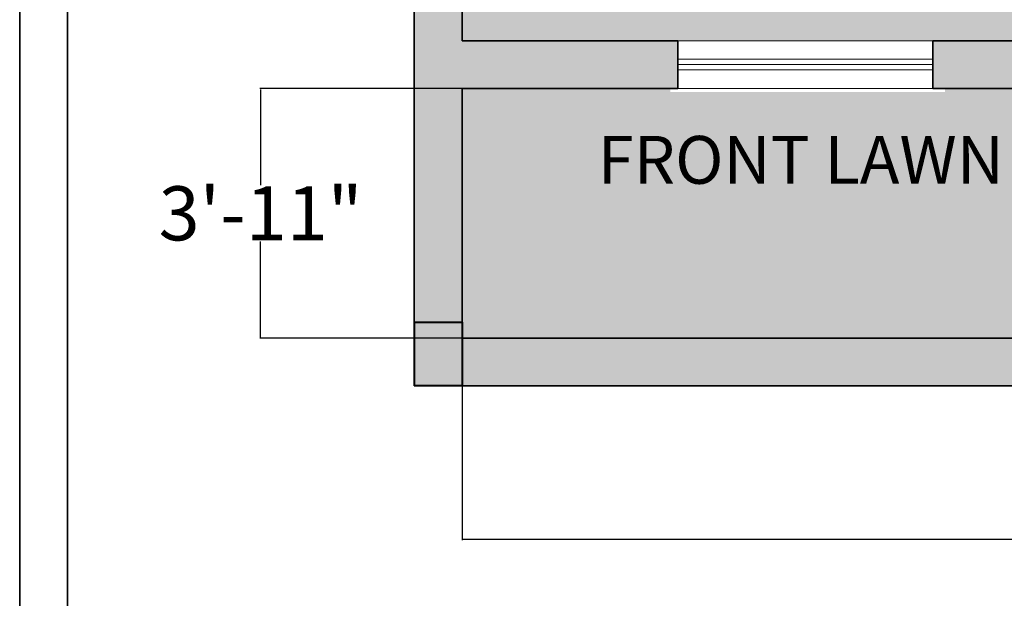
# Model space of a CAD drawing. Units: inches. Extents: x 1077 to 2505, y 1892 to 2728.
# Tile 2 of 26: x 1104 to 1290, y 2048 to 2157. Entities that reach past the tile are written whole.
import ezdxf

# ---------------------------------------------------------------- set-up
doc = ezdxf.new("R2010")
doc.units = ezdxf.units.IN
doc.linetypes.add('ACAD_ISO02W100', pattern=[15, 12, -3])
doc.layers.get('Defpoints').update_dxf_attribs({"color": 220, "linetype": 'ACAD_ISO02W100'})
for name, color, linetype, lineweight in [('A-ANNO-DIMS', 2, 'Continuous', 18), ('A-ANNO-TTLB', 7, 'Continuous', 35), ('A-AREA-IDEN', 7, 'Continuous', 18), ('A-COLS', 7, 'Continuous', 40), ('A-WALL-PATT', 7, 'Continuous', 9), ('WALL', 7, 'Continuous', 35), ('WINDOW', 160, 'Continuous', 13)]:
    doc.layers.add(name, color=color, linetype=linetype, lineweight=lineweight)
doc.layers.add('A-FLOR-PATT', color=254, linetype='Continuous', lineweight=9, true_color=0xd7ebd2)
doc.layers.add('L-PLNT-PATT', color=116, linetype='Continuous', lineweight=9, true_color=0x136734)
doc.styles.get("Standard").update_dxf_attribs({"font": 'arial.ttf'})
doc.dimstyles.get("Standard").update_dxf_attribs({"dimtxt": 10.18, "dimasz": 0.18, "dimexe": 0.18, "dimexo": 0.0625, "dimgap": 0.09, "dimtad": 0, "dimtih": 1, "dimtoh": 1, "dimdec": 0, "dimzin": 0, "dimdsep": 46, "dimlunit": 3, "dimtxsty": 'Standard', "dimcen": 0.09, "dimadec": 0, "dimazin": 0, "dimtfac": 1, "dimtdec": 0, "dimtofl": 0, "dimtmove": 0, "dimatfit": 3, "dimfxl": 1, "dimtolj": 1, "dimtzin": 0, "dimarcsym": 0})

# ---------------------------------------------------------------- blocks, each defined once
blk = doc.blocks.new('C1')
h = blk.add_hatch(color=256)
h.dxf.hatch_style = 1
h.paths.add_polyline_path([(1668.56, 2445.41), (1677.56, 2445.41), (1677.56, 2457.41), (1668.56, 2457.41)])
for p, q in [((1668.56, 2457.41), (1677.56, 2457.41)), ((1668.56, 2445.41), (1668.56, 2457.41)), ((1677.56, 2457.41), (1677.56, 2445.41)), ((1677.56, 2445.41), (1668.56, 2445.41))]:
    blk.add_line(p, q)
blk = doc.blocks.new('WINDOW-48-EXT')
for p, q in [((0, 48), (0, 0)), ((3.5, 48), (3.5, 0)), ((4.5, 48), (4.5, 0)), ((5.5, 48), (5.5, 0)), ((9, 0), (9, 48))]:
    blk.add_line(p, q)
blk = doc.blocks.new('SHEET-FRAME-RESIDENTIAL')
for points in [[(0, 830.04), (543.52, 830.04), (543.52, 0), (0, 0)], [(9, 821.04), (534.52, 821.04), (534.52, 9), (9, 9)]]:
    blk.add_lwpolyline(points, close=True)
blk = doc.blocks.new('*D65')
at = {"layer": 'A-ANNO-DIMS', "color": 0, "lineweight": -2, "transparency": 16777216}
for p, q in [((1187.53, 2097.1), (1187.53, 2059.13)), ((1432.53, 2097.1), (1432.53, 2059.13)), ((1187.71, 2059.31), (1292.37, 2059.31)), ((1432.35, 2059.31), (1327.69, 2059.31))]:
    blk.add_line(p, q, dxfattribs=at)
at = {"layer": 'A-ANNO-DIMS', "color": 0, "transparency": 16777216}
for points in [[(1187.71, 2059.34), (1187.71, 2059.28), (1187.53, 2059.31)], [(1432.35, 2059.34), (1432.35, 2059.28), (1432.53, 2059.31)]]:
    blk.add_solid(points, dxfattribs=at)
at = {"layer": 'Defpoints', "color": 0, "transparency": 16777216}
for p in [(1187.53, 2097.16), (1432.53, 2097.16), (1432.53, 2059.31)]:
    blk.add_point(p, dxfattribs=at)
at = {"layer": 'A-ANNO-DIMS', "color": 0, "transparency": 16777216, "insert": (1310.03, 2059.31), "char_height": 10.18, "attachment_point": 5}
blk.add_mtext('\\A1;20\'-5"', dxfattribs=at)
blk = doc.blocks.new('*D66')
at = {"layer": 'A-ANNO-DIMS', "color": 0, "lineweight": -2, "transparency": 16777216}
for p, q in [((1187.47, 2144.16), (1149.43, 2144.16)), ((1149.61, 2143.98), (1149.61, 2125.95)), ((1149.61, 2097.34), (1149.61, 2115.37)), ((1187.47, 2097.16), (1149.43, 2097.16))]:
    blk.add_line(p, q, dxfattribs=at)
at = {"layer": 'A-ANNO-DIMS', "color": 0, "transparency": 16777216}
for points in [[(1149.58, 2143.98), (1149.64, 2143.98), (1149.61, 2144.16)], [(1149.58, 2097.34), (1149.64, 2097.34), (1149.61, 2097.16)]]:
    blk.add_solid(points, dxfattribs=at)
at = {"layer": 'Defpoints', "color": 0, "transparency": 16777216}
for p in [(1149.61, 2144.16), (1187.53, 2144.16), (1187.53, 2097.16)]:
    blk.add_point(p, dxfattribs=at)
at = {"layer": 'A-ANNO-DIMS', "color": 0, "transparency": 16777216, "insert": (1149.61, 2120.66), "char_height": 10.18, "attachment_point": 5}
blk.add_mtext('\\A1;3\'-11"', dxfattribs=at)

msp = doc.modelspace()

# ---------------------------------------------------------------- hatches: boundary and pattern name
at = {"layer": 'A-FLOR-PATT', "transparency": 33554559}
h = msp.add_hatch(color=256, dxfattribs=at)
h.dxf.hatch_style = 1
h.paths.add_polyline_path([(1395.53, 2577.16), (1374.83, 2577.16), (1350.83, 2577.19), (1350.83, 2577.16), (1329.53, 2577.16), (1329.53, 2480.16), (1329.53, 2469.16), (1325.53, 2469.16), (1325.53, 2515.13), (1307.53, 2515.13), (1307.53, 2577.16), (1269.31, 2577.16), (1221.31, 2577.15), (1221.31, 2577.16), (1187.53, 2577.16), (1187.53, 2433.16), (1289.53, 2433.16), (1289.53, 2429.16), (1263.53, 2429.16), (1187.53, 2429.16), (1187.53, 2395.02), (1187.53, 2395.02), (1187.53, 2371.02), (1187.53, 2371.02), (1187.53, 2307.16), (1259.53, 2307.16), (1259.53, 2399.16), (1263.53, 2399.16), (1263.53, 2307.16), (1289.53, 2307.16), (1289.53, 2306.23), (1325.53, 2306.23), (1325.53, 2307.16), (1329.53, 2307.16), (1329.53, 2306.23), (1365.53, 2306.23), (1365.53, 2307.16), (1432.53, 2307.16), (1432.53, 2088.16), (1547.53, 2088.16), (1547.53, 2140.08), (1511.53, 2140.08), (1511.53, 2267.16), (1475.53, 2267.16), (1475.53, 2303.16), (1468.53, 2303.16), (1468.53, 2307.16), (1547.53, 2307.16), (1547.53, 2348.22), (1547.53, 2396.22), (1547.53, 2429.16), (1435.53, 2429.16), (1435.53, 2433.16), (1476.35, 2433.16), (1476.35, 2451.18), (1547.53, 2451.18), (1547.53, 2577.16), (1499.53, 2577.16), (1499.53, 2586.16), (1547.53, 2586.16), (1547.53, 2642.16), (1518.18, 2642.16), (1518.18, 2642.05), (1494.15, 2642.05), (1494.15, 2642.16), (1469.53, 2642.16), (1469.53, 2577.16), (1399.53, 2577.16), (1399.53, 2429.16), (1325.53, 2429.16), (1325.53, 2433.16), (1329.53, 2433.16), (1395.53, 2433.16), (1395.53, 2480.16), (1359.53, 2480.16), (1359.53, 2484.16), (1395.53, 2484.16)])
h.paths.add_polyline_path([(1357.65, 2482.07), (1355.65, 2482.07), (1355.65, 2481.07, 0.414214), (1356.65, 2480.07), (1344.65, 2480.07), (1344.65, 2477.06), (1343.27, 2477.06), (1343.27, 2480.07), (1330.65, 2480.07, -0.414214), (1329.65, 2481.07), (1329.65, 2484.07), (1331.65, 2484.07), (1331.65, 2510.07, -0.446908)], flags=16)
h.paths.add_polyline_path([(1305.09, 2559.18), (1288.89, 2559.18), (1288.89, 2575.38), (1305.09, 2575.38)], flags=16)
h.paths.add_polyline_path([(1304.19, 2560.08), (1289.79, 2560.08), (1289.79, 2574.48), (1304.19, 2574.48)], flags=0)
h.paths.add_polyline_path([(1287.99, 2500.68, -0.414214), (1287.09, 2499.78), (1265.14, 2499.78), (1224.09, 2499.78, -0.414214), (1223.19, 2500.68), (1223.19, 2557.16), (1223.19, 2571.74), (1223.19, 2575.38), (1287.99, 2575.38), (1287.99, 2571.74), (1287.09, 2571.74, -0.414214), (1287.99, 2570.84)], flags=16)
h.paths.add_polyline_path([(1292.98, 2569.05, -1), (1300.92, 2569.05, -1)], flags=0)
h.paths.add_polyline_path([(1293.32, 2569.05, -1), (1300.58, 2569.05, -1)], flags=0)
h.paths.add_polyline_path([(1322.8, 2462.21), (1322.8, 2431.71), (1323.05, 2430.71), (1323.05, 2431.71), (1321.8, 2431.71), (1321.8, 2462.19, 0.404641), (1292.3, 2431.71), (1292.05, 2430.71, -0.414214), (1291.55, 2430.21), (1291.05, 2430.21), (1291.05, 2429.71, -0.414214), (1290.55, 2429.21), (1289.55, 2429.21), (1289.55, 2434.21), (1290.55, 2434.21, -0.414214), (1291.05, 2433.71), (1291.05, 2433.21), (1291.55, 2433.21, -0.414214), (1292.05, 2432.71), (1292.3, 2431.71, -0.414214)], flags=16)
h.paths.add_polyline_path([(1287.82, 2548.28, 0.292232), (1279.17, 2536.8, 0.052719), (1223.93, 2548.28), (1223.28, 2548.28), (1223.28, 2557.16), (1223.93, 2557.16), (1245.42, 2557.16, -0.117785), (1245.77, 2557.93, -0.059418), (1254.87, 2567.02, -0.379859), (1257.28, 2566.88, -0.02509), (1261.41, 2563.32, -0.025935), (1265.65, 2567.02, -0.379859), (1268.06, 2566.88, -0.061767), (1277.52, 2557.43, -0.069393), (1277.82, 2557.16), (1287.82, 2557.16)], flags=0)
h.paths.add_polyline_path([(1263.47, 2548.28), (1260.56, 2548.28, -0.015371), (1258.01, 2546.13, -0.429576), (1255.37, 2546.06, -0.016036), (1252.69, 2548.28), (1223.28, 2548.28), (1223.28, 2554.42), (1246.78, 2554.42, 0.055344), (1255.37, 2546.06, 0.331768), (1257.52, 2545.74, 0.027343), (1262, 2549.64, 0.00919)], flags=0)
h.paths.add_polyline_path([(1295.56, 2568.34), (1296.87, 2569.09), (1296.87, 2570.6, 0.399698), (1295.39, 2569.05, 0.119004)], flags=0)
h.paths.add_polyline_path([(1295.21, 2569.05, -1), (1298.68, 2569.05, -1)], flags=0)
h.paths.add_polyline_path([(1296.95, 2568.96), (1297.03, 2569), (1297.03, 2569.09), (1296.99, 2569.11), (1296.91, 2568.98)], flags=0)
h.paths.add_polyline_path([(1402.28, 2462.19, -0.414214), (1432.78, 2431.69), (1433.03, 2432.69), (1432.78, 2431.69, 0.404641), (1403.28, 2462.17), (1403.28, 2431.69), (1402.03, 2431.69), (1402.03, 2430.69, -0.414214), (1401.53, 2430.19), (1401.03, 2430.19), (1401.03, 2429.69, -0.414214), (1400.53, 2429.19), (1399.53, 2429.19), (1399.53, 2434.19), (1400.53, 2434.19, -0.414214), (1401.03, 2433.69), (1401.03, 2433.19), (1401.53, 2433.19, -0.414214), (1402.03, 2432.69)], flags=16)
h.paths.add_polyline_path([(1470.16, 2535.21, -0.414214), (1471.06, 2536.11), (1527.54, 2536.11), (1542.12, 2536.11), (1545.76, 2536.11), (1545.76, 2471.31), (1542.12, 2471.31), (1542.12, 2472.21, -0.414214), (1541.22, 2471.31), (1471.06, 2471.31, -0.414214), (1470.16, 2472.21), (1470.16, 2494.16)], flags=16)
h.paths.add_polyline_path([(1483.07, 2536.11, 0.253465), (1480.11, 2526.15, 0.2538), (1470.15, 2523.19)], flags=16)
h.paths.add_polyline_path([(1223.19, 2512.69, 0.253465), (1233.14, 2509.74, 0.2538), (1236.1, 2499.77)], flags=16)
h.paths.add_polyline_path([(1469.77, 2578.72), (1469.77, 2581.72), (1471.77, 2581.72), (1471.77, 2607.72, -0.01951), (1473.77, 2607.68), (1473.77, 2579.72), (1473.77, 2578.72, -0.414214), (1472.77, 2577.72), (1470.77, 2577.72, -0.414214)], flags=16)
h.paths.add_polyline_path([(1382.46, 2398.13), (1395.04, 2398.13), (1395.04, 2399.74), (1382.46, 2399.74)], flags=16)
h.paths.add_polyline_path([(1379.94, 2397.18), (1379.94, 2389.82), (1380.5, 2389.82), (1380.5, 2396.05, -0.41429), (1381.06, 2396.61), (1396.47, 2396.61, -0.414213), (1397.03, 2396.05), (1397.03, 2389.82), (1397.59, 2389.82), (1397.59, 2397.18)], flags=16)
h.paths.add_polyline_path([(1263.37, 2428.14), (1263.37, 2426.14, -0.414214), (1262.37, 2425.14), (1261.37, 2425.14), (1233.41, 2425.14, 0.400854), (1259.37, 2401.04), (1259.37, 2401.14), (1261.37, 2401.14, -0.446908), (1233.37, 2427.14), (1259.37, 2427.14), (1259.37, 2429.14), (1262.37, 2429.14, -0.414214)], flags=16)
h.paths.add_polyline_path([(1404.79, 2398.13), (1417.37, 2398.13), (1417.37, 2399.74), (1404.79, 2399.74)], flags=16)
h.paths.add_polyline_path([(1402.27, 2397.18), (1404.79, 2398.13), (1417.37, 2398.13), (1419.92, 2397.18)], flags=16)
h.paths.add_polyline_path([(1432.26, 2383.16), (1432.26, 2370.59), (1433.87, 2370.59), (1433.87, 2383.16)], flags=16)
h.paths.add_polyline_path([(1431.3, 2385.69), (1423.84, 2385.69), (1423.84, 2385.13), (1430.18, 2385.13, -0.41429), (1430.74, 2384.57), (1430.74, 2369.16, -0.414237), (1430.18, 2368.6), (1423.84, 2368.6), (1423.84, 2368.03), (1431.3, 2368.03)], flags=16)
h.paths.add_polyline_path([(1417.37, 2351.16), (1417.37, 2349.54), (1418.9, 2349.54, 0.414236), (1419.92, 2350.56), (1419.92, 2352.11)], flags=16)
h.paths.add_polyline_path([(1395.04, 2351.16), (1395.04, 2349.54), (1396.58, 2349.54, 0.414235), (1397.59, 2350.56), (1397.59, 2352.11)], flags=16)
h.paths.add_polyline_path([(1366.7, 2370.05), (1365.09, 2370.05), (1365.09, 2368.52, 0.414235), (1366.11, 2367.5), (1367.66, 2367.5)], flags=16)
h.paths.add_polyline_path([(1419.36, 2359.47), (1419.36, 2353.24, -0.41419), (1418.8, 2352.68), (1403.39, 2352.68, -0.414137), (1402.83, 2353.24), (1402.83, 2359.47), (1397.03, 2359.47), (1397.03, 2353.24, -0.414189), (1396.47, 2352.68), (1381.06, 2352.68, -0.414137), (1380.5, 2353.24), (1380.5, 2359.47)], flags=16)
h.paths.add_polyline_path([(1222.29, 2559.18), (1206.09, 2559.18), (1206.09, 2575.38), (1222.29, 2575.38)], flags=16)
h.paths.add_polyline_path([(1221.39, 2560.08), (1206.99, 2560.08), (1206.99, 2574.48), (1221.39, 2574.48)], flags=0)
h.paths.add_polyline_path([(1482, 2577.72), (1482, 2580.73), (1483.38, 2580.73), (1483.38, 2577.72), (1484.77, 2577.72), (1484.77, 2574.72), (1483.38, 2574.72), (1483.38, 2577.72)], flags=16)
h.paths.add_polyline_path([(1266.37, 2415.53), (1266.37, 2414.14), (1263.37, 2414.14), (1263.37, 2415.53), (1260.36, 2415.53), (1260.36, 2416.91), (1263.37, 2416.91), (1263.37, 2415.53)], flags=16)
h.paths.add_polyline_path([(1210.26, 2569.05, -1), (1218.19, 2569.05, -1)], flags=0)
h.paths.add_polyline_path([(1210.6, 2569.05, -1), (1217.85, 2569.05, -1)], flags=0)
h.paths.add_polyline_path([(1212.84, 2568.34), (1214.15, 2569.09), (1214.15, 2570.6, 0.399698), (1212.67, 2569.05, 0.119004)], flags=0)
h.paths.add_polyline_path([(1212.49, 2569.05, -1), (1215.96, 2569.05, -1)], flags=0)
h.paths.add_polyline_path([(1214.23, 2568.96), (1214.3, 2568.91), (1214.3, 2569)], flags=0)
h.paths.add_polyline_path([(1507.18, 2480.12, 0.052719), (1518.66, 2535.36), (1518.66, 2536.01), (1527.54, 2536.01), (1527.54, 2535.36), (1527.54, 2513.88, -0.117785), (1528.31, 2513.53, -0.059418), (1537.4, 2504.43, -0.379859), (1537.26, 2502.01, -0.02509), (1533.7, 2497.89, -0.025935), (1537.4, 2493.64, -0.379859), (1537.26, 2491.23, -0.061767), (1527.8, 2481.77, -0.069393), (1527.54, 2481.47), (1527.54, 2471.47), (1518.66, 2471.47, 0.292232)], flags=0)
h.paths.add_polyline_path([(1516.43, 2503.92, -0.016036), (1518.66, 2506.6), (1518.66, 2536.01), (1524.8, 2536.01), (1524.8, 2512.51, 0.055344), (1516.43, 2503.92, 0.331768), (1516.12, 2501.77, 0.027343), (1520.01, 2497.29, 0.00919), (1518.66, 2495.82), (1518.66, 2498.73, -0.015371), (1516.5, 2501.28, -0.429576)], flags=0)
h.paths.add_polyline_path([(1499.63, 2625.5, -0.171636), (1502.82, 2631.01), (1502.82, 2633.37), (1498.68, 2633.37, -0.414214), (1497.7, 2634.36), (1497.7, 2640.66, -0.414214), (1498.68, 2641.64), (1514.82, 2641.64, -0.414214), (1515.81, 2640.66), (1515.81, 2634.36, -0.414214), (1514.82, 2633.37), (1510.69, 2633.37), (1510.69, 2631.01, -0.171636), (1513.88, 2625.5, -0.258205), (1509.31, 2614.47), (1504.19, 2614.47, -0.258205)], flags=16)
h.paths.add_polyline_path([(1501.2, 2625.5, -0.171636), (1504.39, 2631.01), (1509.12, 2631.01, -0.171636), (1512.3, 2625.5, -0.210384), (1509.35, 2616.02), (1504.16, 2616.02, -0.210384)], flags=0)
h.paths.add_polyline_path([(1529.56, 2537.01), (1529.56, 2553.21), (1545.76, 2553.21), (1545.76, 2537.01)], flags=16)
h.paths.add_polyline_path([(1530.46, 2537.91), (1530.46, 2552.31), (1544.86, 2552.31), (1544.86, 2537.91)], flags=0)
h.paths.add_polyline_path([(1535.45, 2545.07, -1), (1543.39, 2545.07, -1)], flags=0)
h.paths.add_polyline_path([(1535.8, 2545.07, -1), (1543.05, 2545.07, -1)], flags=0)
h.paths.add_polyline_path([(1529.56, 2470.41), (1545.76, 2470.41), (1545.76, 2454.21), (1529.56, 2454.21)], flags=16)
h.paths.add_polyline_path([(1541.16, 2544.99), (1540.98, 2544.99, -0.544606), (1538.71, 2543.68), (1538.62, 2543.53, 0.547962)], flags=0)
h.paths.add_polyline_path([(1530.46, 2469.51), (1544.86, 2469.51), (1544.86, 2455.11), (1530.46, 2455.11)], flags=0)
h.paths.add_polyline_path([(1539.47, 2545.14), (1539.42, 2545.22), (1539.38, 2545.14)], flags=0)
h.paths.add_polyline_path([(1543.39, 2462.34, -1), (1535.45, 2462.34, -1)], flags=0)
h.paths.add_polyline_path([(1543.05, 2462.34, -1), (1535.8, 2462.34, -1)], flags=0)
h.paths.add_polyline_path([(1541.16, 2462.27), (1540.98, 2462.27, -0.544606), (1538.71, 2460.96), (1538.62, 2460.8, 0.547962)], flags=0)
h.paths.add_polyline_path([(1539.47, 2462.42), (1539.42, 2462.5), (1539.38, 2462.42)], flags=0)
h.paths.add_polyline_path([(1435.32, 2335.25, -0.414214), (1465.82, 2304.75), (1466.07, 2305.75), (1465.82, 2304.75, 0.404641), (1436.32, 2335.23), (1436.32, 2304.75), (1435.07, 2304.75), (1435.07, 2303.75, -0.414214), (1434.57, 2303.25), (1434.07, 2303.25), (1434.07, 2302.75, -0.414214), (1433.57, 2302.25), (1432.57, 2302.25), (1432.57, 2307.25), (1433.57, 2307.25, -0.414214), (1434.07, 2306.75), (1434.07, 2306.25), (1434.57, 2306.25, -0.414214), (1435.07, 2305.75)], flags=16)
h.paths.add_polyline_path([(1532.13, 2635.71), (1535.43, 2635.71), (1535.43, 2635.89), (1532.13, 2635.89)], flags=16)
edge = h.paths.add_edge_path(flags=16)
edge.add_arc((1535.98, 2632.67), 0.183, 270, 360)
edge.add_line((1536.17, 2632.67), (1536.17, 2639.82))
edge.add_line((1536.17, 2639.82), (1538.29, 2639.82))
edge.add_line((1538.29, 2639.82), (1538.29, 2641.82))
edge.add_line((1538.29, 2641.82), (1533.25, 2641.82))
edge.add_line((1533.25, 2641.82), (1533.25, 2639.82))
edge.add_line((1533.25, 2639.82), (1534.87, 2639.82))
edge.add_line((1534.87, 2639.82), (1534.87, 2639))
edge.add_line((1534.87, 2639), (1533.7, 2639))
edge.add_line((1533.7, 2639), (1533.7, 2639.82))
edge.add_line((1533.7, 2639.82), (1533.25, 2639.82))
edge.add_line((1533.25, 2639.82), (1533.25, 2641.82))
edge.add_line((1533.25, 2641.82), (1538.29, 2641.82))
edge.add_line((1538.29, 2641.82), (1538.29, 2641.34))
edge.add_line((1538.29, 2641.34), (1540.64, 2641.58))
edge.add_line((1540.64, 2641.58), (1540.64, 2641.82))
edge.add_line((1540.64, 2641.82), (1541.5, 2641.82))
edge.add_line((1541.5, 2641.82), (1541.5, 2641.25))
edge.add_line((1541.5, 2641.25), (1541.31, 2639.79))
edge.add_ellipse((1541.09, 2638.95), major_axis=(-1.08, 0), ratio=0.790849, start_angle=180, end_angle=255.2976, ccw=False)
edge.add_line((1542.17, 2638.95), (1542.17, 2638.38))
edge.add_ellipse((1541.09, 2638.38), major_axis=(-1.08, 0), ratio=0.790849, start_angle=0, end_angle=180, ccw=False)
edge.add_line((1540, 2638.38), (1540.01, 2638.87))
edge.add_ellipse((1541.09, 2638.95), major_axis=(-1.08, 0), ratio=0.790849, start_angle=284.7024, end_angle=364.0401, ccw=False)
edge.add_line((1540.78, 2639.75), (1540.78, 2641.25))
edge.add_line((1540.78, 2641.25), (1540.64, 2641.25))
edge.add_line((1540.64, 2641.25), (1538.29, 2641.01))
edge.add_line((1538.29, 2641.01), (1538.29, 2639.82))
edge.add_line((1538.29, 2639.82), (1536.17, 2639.82))
edge.add_line((1536.17, 2639.82), (1536.17, 2632.48))
edge.add_line((1536.17, 2632.48), (1535.98, 2632.48))
h.paths.add_polyline_path([(1496.32, 2250.34, -0.292371), (1498.9, 2247.83, -0.085148), (1501.21, 2208.85, -0.01331), (1500.27, 2098.5, -0.379287), (1497.22, 2095.28, -0.0502), (1441.54, 2095.28, -0.379287), (1438.5, 2098.5, -0.01331), (1437.56, 2208.85, -0.086132), (1439.96, 2248.26, -0.295116), (1442.59, 2250.78, -0.114238)], flags=16)
h.paths.add_polyline_path([(1495.16, 2205.84, -0.355389), (1496.7, 2202.1), (1492.94, 2189.65, -0.398275), (1489.12, 2187.47, 0.113332), (1449.64, 2187.47, -0.398275), (1445.82, 2189.65), (1442.06, 2202.1, -0.355394), (1443.6, 2205.84, -0.265725)], flags=0)
h.paths.add_polyline_path([(1440.37, 2195.72), (1445.94, 2181.67), (1445.94, 2160.63), (1440.84, 2157.26)], flags=0)
h.paths.add_polyline_path([(1498.46, 2195.72), (1497.99, 2157.26), (1492.88, 2160.63), (1492.88, 2181.67)], flags=0)
h.paths.add_polyline_path([(1445.94, 2158.37), (1445.94, 2137.12), (1441.12, 2122.56), (1440.87, 2155.03)], flags=0)
h.paths.add_polyline_path([(1492.88, 2158.37), (1497.96, 2155.03), (1497.71, 2122.56), (1492.88, 2137.12)], flags=0)
h.paths.add_polyline_path([(1489.88, 2130.4), (1494.39, 2107.67, -0.090102), (1444.44, 2107.65), (1448.95, 2130.39, 0.036636)], flags=0)
h.paths.add_polyline_path([(1447.54, 2159.34), (1497.44, 2159.34), (1497.44, 2177.89), (1447.54, 2177.89)], flags=8)
h.paths.add_polyline_path([(1196.44, 2354.84), (1246.65, 2354.84), (1246.65, 2388.43), (1196.44, 2388.43)], flags=24)
h.paths.add_polyline_path([(1296.09, 2360.25), (1353.81, 2360.25), (1353.81, 2393.84), (1296.09, 2393.84)], flags=24)
h.paths.add_polyline_path([(1400.72, 2471.85), (1470.63, 2471.85), (1470.63, 2505.44), (1400.72, 2505.44)], flags=24)
h.paths.add_polyline_path([(1324.78, 2448.48), (1394.95, 2448.48), (1394.95, 2467.02), (1324.78, 2467.02)], flags=24)
h.paths.add_polyline_path([(1335.08, 2531.43), (1389.67, 2531.43), (1389.67, 2565.02), (1335.08, 2565.02)], flags=24)
h.paths.add_polyline_path([(1225.76, 2460), (1295.67, 2460), (1295.67, 2493.58), (1225.76, 2493.58)], flags=24)
h = msp.add_hatch(color=256, dxfattribs=at)
h.dxf.hatch_style = 1
h.paths.add_polyline_path([(1547.53, 2348.22), (1547.53, 2396.22), (1547.53, 2425.11), (1547.53, 2425.11), (1547.53, 2429.16), (1435.53, 2429.16), (1434.03, 2429.21), (1434.03, 2430.19), (1433.03, 2430.19), (1432.78, 2431.69, 0.404641), (1403.28, 2462.17), (1403.28, 2431.69), (1402.03, 2431.69), (1402.03, 2430.19), (1401.03, 2430.19), (1401.03, 2429.19), (1399.53, 2429.19), (1399.53, 2429.19), (1399.53, 2429.16), (1334.67, 2429.16), (1334.67, 2423.95), (1325.67, 2423.95), (1325.67, 2429.16), (1325.53, 2429.16), (1324.05, 2429.24), (1324.05, 2430.21), (1323.05, 2430.21), (1323.05, 2431.71), (1321.8, 2431.71), (1321.8, 2462.19, 0.416544), (1292.05, 2430.73, -0.423614), (1291.55, 2430.21), (1291.05, 2430.21), (1291.05, 2429.21), (1289.55, 2429.21), (1289.53, 2429.21), (1289.53, 2429.16), (1263.37, 2429.16), (1263.37, 2415.53), (1266.37, 2415.53), (1266.37, 2414.14), (1263.37, 2414.14), (1263.37, 2399.16), (1263.53, 2399.16), (1263.53, 2307.16), (1289.53, 2307.16), (1289.53, 2306.23), (1323.26, 2306.23), (1323.26, 2307.21), (1332.26, 2307.21), (1365.53, 2306.23), (1365.53, 2307.16), (1432.53, 2307.16), (1432.57, 2307.16), (1432.57, 2307.25), (1434.07, 2307.25), (1434.07, 2306.25), (1435.32, 2306.25), (1435.32, 2335.25, -0.407346), (1466.07, 2305.73, -0.423614), (1466.57, 2306.25), (1467.07, 2306.25), (1467.07, 2307.25), (1468.57, 2307.25), (1547.53, 2307.16), (1547.53, 2307.2)])
h.paths.add_polyline_path([(1430.74, 2369.16), (1430.74, 2384.57, 0.41429), (1430.18, 2385.13), (1423.84, 2385.13), (1423.84, 2368.6), (1430.18, 2368.6, 0.414237)], flags=16)
h.paths.add_polyline_path([(1432.26, 2383.16), (1432.26, 2370.59), (1433.87, 2370.59), (1433.87, 2383.16)], flags=16)
h.paths.add_polyline_path([(1431.3, 2368.03), (1431.3, 2385.69), (1432.26, 2383.16), (1432.26, 2370.59)], flags=16)
h.paths.add_polyline_path([(1417.37, 2351.16), (1417.37, 2349.54), (1418.9, 2349.54, 0.414236), (1419.92, 2350.56), (1419.92, 2352.11)], flags=16)
h.paths.add_polyline_path([(1403.39, 2352.68), (1418.78, 2352.68, 0.42427), (1419.36, 2353.24), (1419.36, 2359.47), (1402.83, 2359.47), (1402.83, 2353.24, 0.414137)], flags=16)
h.paths.add_polyline_path([(1366.7, 2370.05), (1365.09, 2370.05), (1365.09, 2368.52, 0.414235), (1366.11, 2367.5), (1367.66, 2367.5)], flags=16)
h.paths.add_polyline_path([(1382.46, 2398.13), (1395.04, 2398.13), (1395.04, 2399.74), (1382.46, 2399.74)], flags=16)
h.paths.add_polyline_path([(1396.47, 2396.61), (1381.06, 2396.61, 0.41429), (1380.5, 2396.05), (1380.5, 2389.82), (1397.03, 2389.82), (1397.03, 2396.05, 0.414213)], flags=16)
h.paths.add_polyline_path([(1402.27, 2397.18), (1402.83, 2396.05, -0.414213), (1403.39, 2396.61)], flags=16)
h.paths.add_polyline_path([(1418.8, 2396.61), (1419.36, 2396.61), (1419.36, 2396.05, 0.414237)], flags=16)
h.paths.add_polyline_path([(1404.79, 2398.13), (1417.37, 2398.13), (1417.37, 2399.74), (1404.79, 2399.74)], flags=16)
h.paths.add_polyline_path([(1381.06, 2352.68, -0.414213), (1380.5, 2353.24), (1380.27, 2352.11)], flags=16)
h.paths.add_polyline_path([(1396.58, 2349.54), (1396.58, 2349.54), (1395.04, 2349.54), (1395.04, 2349.54), (1382.46, 2349.54), (1382.46, 2351.16), (1395.04, 2351.16), (1397.59, 2352.11), (1397.59, 2350.56, -0.414235)], flags=16)
h.paths.add_polyline_path([(1379.94, 2397.18), (1382.46, 2398.13), (1395.04, 2398.13), (1397.59, 2397.18)], flags=16)
h.paths.add_polyline_path([(1368.78, 2384.59, 0.414213), (1368.22, 2384.03), (1367.66, 2367.5), (1367.66, 2385.15)], flags=16)
h.paths.add_polyline_path([(1547.53, 2574.38), (1547.51, 2574.38), (1547.51, 2577.16), (1499.53, 2577.16), (1484.77, 2577.44), (1484.77, 2574.72), (1483.38, 2574.72), (1483.38, 2577.72), (1482, 2577.72), (1469.53, 2577.72), (1469.53, 2577.16), (1401.95, 2577.16), (1401.95, 2574.12), (1399.53, 2574.12), (1399.53, 2434.19), (1401.03, 2434.19), (1401.03, 2433.19), (1402.28, 2433.19), (1402.28, 2462.19, -0.407346), (1433.03, 2432.67, -0.423614), (1433.53, 2433.19), (1434.03, 2433.19), (1434.03, 2434.19), (1435.53, 2434.19), (1476.35, 2433.81), (1476.35, 2451.18), (1547.53, 2451.18)])
h.paths.add_polyline_path([(1470.16, 2535.21, -0.414214), (1471.06, 2536.11), (1527.54, 2536.11), (1542.12, 2536.11), (1545.76, 2536.11), (1545.76, 2471.31), (1542.12, 2471.31), (1542.12, 2472.21, -0.414214), (1541.22, 2471.31), (1471.06, 2471.31, -0.414214), (1470.16, 2472.21), (1470.16, 2494.16)], flags=16)
h.paths.add_polyline_path([(1483.07, 2536.11, 0.253465), (1480.11, 2526.15, 0.2538), (1470.15, 2523.19)], flags=16)
h.paths.add_polyline_path([(1525.55, 2481.52, -0.000893), (1524.8, 2482.24), (1524.8, 2471.47), (1527.54, 2471.47), (1527.54, 2472.12), (1527.54, 2481.47, -0.388819)], flags=0)
h.paths.add_polyline_path([(1518.66, 2536.01), (1527.54, 2536.01), (1527.54, 2535.36), (1527.54, 2513.88, -0.117785), (1528.31, 2513.53, -0.059418), (1537.4, 2504.43, -0.379859), (1537.26, 2502.01, -0.02509), (1533.7, 2497.89, 0.033431), (1528.3, 2502.74, 0.308459), (1526.25, 2502.88, 0.047827), (1518.66, 2495.82), (1518.66, 2498.73, -0.015371), (1516.5, 2501.28, -0.429576), (1516.43, 2503.92, -0.016036), (1518.66, 2506.6)], flags=0)
h.paths.add_polyline_path([(1529.56, 2537.01), (1529.56, 2553.21), (1545.76, 2553.21), (1545.76, 2537.01)], flags=16)
h.paths.add_polyline_path([(1530.46, 2537.91), (1530.46, 2552.31), (1544.86, 2552.31), (1544.86, 2537.91)], flags=0)
h.paths.add_polyline_path([(1535.8, 2545.07, -1), (1543.05, 2545.07, -1)], flags=0)
h.paths.add_polyline_path([(1541.16, 2544.99), (1540.98, 2544.99, -0.544606), (1538.71, 2543.68), (1538.62, 2543.53, 0.547962)], flags=0)
h.paths.add_polyline_path([(1539.47, 2545.14), (1539.42, 2545.22), (1539.38, 2545.14)], flags=0)
h.paths.add_polyline_path([(1529.56, 2470.41), (1545.76, 2470.41), (1545.76, 2454.21), (1529.56, 2454.21)], flags=16)
h.paths.add_polyline_path([(1530.46, 2469.51), (1544.86, 2469.51), (1544.86, 2455.11), (1530.46, 2455.11)], flags=0)
h.paths.add_polyline_path([(1535.8, 2462.34, -1), (1543.05, 2462.34, -1)], flags=0)
h.paths.add_polyline_path([(1541.16, 2462.27), (1540.98, 2462.27, -0.544606), (1538.71, 2460.96), (1538.62, 2460.8, 0.547962)], flags=0)
h.paths.add_polyline_path([(1539.47, 2462.42), (1539.42, 2462.5), (1539.38, 2462.42)], flags=0)
h.paths.add_polyline_path([(1395.53, 2574.12), (1392.95, 2574.12), (1392.95, 2577.16), (1374.83, 2577.16), (1350.83, 2577.19), (1350.83, 2577.16), (1332.07, 2577.16), (1332.07, 2574), (1329.53, 2574), (1329.53, 2484.07), (1331.65, 2484.07), (1331.65, 2510.07, -0.423677), (1357.76, 2484.07), (1359.53, 2484.07), (1359.53, 2484.16), (1395.53, 2484.16)], flags=17)
h.paths.add_polyline_path([(1395.53, 2480.16), (1359.06, 2480.16, 0.437533), (1359.53, 2481.55), (1359.53, 2484.16), (1395.53, 2484.16), (1395.53, 2574.12), (1392.95, 2574.12), (1392.95, 2577.16), (1374.83, 2577.16), (1350.83, 2577.19), (1350.83, 2577.16), (1332.07, 2577.16), (1332.07, 2574), (1329.53, 2574), (1329.53, 2484.07), (1329.65, 2484.07), (1329.65, 2481.07), (1329.53, 2480.16), (1329.53, 2469.16), (1325.53, 2469.16), (1325.53, 2515.13), (1307.53, 2515.13), (1307.53, 2577.16), (1269.31, 2577.16), (1221.31, 2577.15), (1221.31, 2577.16), (1187.61, 2577.16), (1187.61, 2574.03), (1187.53, 2433.16), (1289.55, 2433.16), (1289.55, 2434.21), (1291.05, 2434.21), (1291.05, 2433.21), (1292.05, 2433.21), (1292.3, 2431.71, -0.414214), (1322.8, 2462.21), (1323.05, 2432.71, -0.414214), (1323.55, 2433.21), (1324.05, 2433.21), (1324.05, 2434.21), (1325.67, 2434.21), (1325.67, 2435.95), (1334.67, 2435.95), (1334.67, 2433.16), (1395.53, 2433.16)])
h.paths.add_polyline_path([(1344.65, 2480.07), (1344.65, 2477.06), (1343.27, 2477.06), (1343.27, 2480.07), (1332.65, 2480.07, 0.414214), (1333.65, 2481.07), (1333.65, 2482.07), (1331.65, 2482.07), (1331.65, 2484.07), (1331.65, 2510.07, -0.446908), (1357.65, 2482.07), (1355.65, 2482.07), (1355.65, 2481.07, 0.414214), (1356.65, 2480.07)], flags=16)
h.paths.add_polyline_path([(1287.99, 2500.68, -0.414214), (1287.09, 2499.78), (1265.14, 2499.78), (1224.09, 2499.78, -0.414214), (1223.19, 2500.68), (1223.19, 2557.16), (1223.19, 2571.74), (1223.19, 2575.38), (1287.99, 2575.38), (1287.99, 2571.74), (1287.09, 2571.74, -0.414214), (1287.99, 2570.84)], flags=16)
h.paths.add_polyline_path([(1277.77, 2555.17, -0.000893), (1277.05, 2554.42), (1287.82, 2554.42), (1287.82, 2557.16), (1287.17, 2557.16), (1277.82, 2557.16, -0.388819)], flags=0)
h.paths.add_polyline_path([(1223.28, 2548.28), (1223.28, 2557.16), (1223.93, 2557.16), (1245.42, 2557.16, -0.117785), (1245.77, 2557.93, -0.059418), (1254.87, 2567.02, -0.379859), (1257.28, 2566.88, -0.02509), (1261.41, 2563.32, 0.033431), (1256.55, 2557.93, 0.308459), (1256.41, 2555.88, 0.047827), (1263.47, 2548.28), (1260.56, 2548.28, -0.015371), (1258.01, 2546.13, -0.429576), (1255.37, 2546.06, -0.016036), (1252.69, 2548.28)], flags=0)
h.paths.add_polyline_path([(1305.09, 2559.18), (1288.89, 2559.18), (1288.89, 2575.38), (1305.09, 2575.38)], flags=16)
h.paths.add_polyline_path([(1304.19, 2560.08), (1289.79, 2560.08), (1289.79, 2574.48), (1304.19, 2574.48)], flags=0)
h.paths.add_polyline_path([(1300.58, 2569.05, -1), (1293.32, 2569.05, -1)], flags=0)
h.paths.add_polyline_path([(1223.19, 2512.69, 0.253465), (1233.14, 2509.74, 0.2538), (1236.1, 2499.77)], flags=16)
h.paths.add_polyline_path([(1295.56, 2568.34), (1296.87, 2569.09), (1296.87, 2570.6, 0.399698), (1295.39, 2569.05, 0.119004)], flags=0)
h.paths.add_polyline_path([(1295.21, 2569.05, -1), (1298.68, 2569.05, -1)], flags=0)
h.paths.add_polyline_path([(1296.95, 2568.96), (1297.03, 2569), (1297.03, 2569.09), (1296.99, 2569.11), (1296.91, 2568.98)], flags=0)
h.paths.add_polyline_path([(1222.29, 2559.18), (1206.09, 2559.18), (1206.09, 2575.38), (1222.29, 2575.38)], flags=16)
h.paths.add_polyline_path([(1221.39, 2560.08), (1206.99, 2560.08), (1206.99, 2574.48), (1221.39, 2574.48)], flags=0)
h.paths.add_polyline_path([(1217.85, 2569.05, -1), (1210.6, 2569.05, -1)], flags=0)
h.paths.add_polyline_path([(1212.84, 2568.34), (1214.15, 2569.09), (1214.15, 2570.6, 0.399698), (1212.67, 2569.05, 0.119004)], flags=0)
h.paths.add_polyline_path([(1212.49, 2569.05, -1), (1215.96, 2569.05, -1)], flags=0)
h.paths.add_polyline_path([(1214.23, 2568.96), (1214.3, 2569), (1214.3, 2569.09), (1214.26, 2569.11), (1214.19, 2568.98)], flags=0)
h.paths.add_polyline_path([(1259.53, 2399.14), (1259.37, 2399.14), (1259.37, 2401.04, -0.423677), (1233.37, 2427.14), (1259.37, 2427.14), (1259.37, 2429.16), (1187.53, 2429.16), (1187.53, 2395.02), (1187.53, 2395.02), (1187.53, 2371.02), (1187.53, 2371.02), (1187.53, 2311.49), (1187.55, 2311.49), (1187.55, 2307.16), (1259.53, 2307.16)])
h.paths.add_polyline_path([(1323.26, 2295.21), (1323.26, 2304.23), (1289.53, 2304.23), (1289.53, 2303.16), (1187.55, 2303.16), (1187.55, 2299.49), (1178.53, 2299.49), (1178.53, 2267.66), (1178.53, 2219.66), (1182.03, 2219.66), (1182.03, 2267.67), (1184.03, 2267.67), (1184.03, 2219.66), (1187.53, 2219.66), (1187.53, 2153.16), (1228.13, 2153.16), (1276.13, 2153.16), (1276.13, 2153.16), (1324.54, 2153.16), (1324.54, 2154.67), (1325.54, 2154.67), (1325.54, 2155.92), (1296.54, 2155.92, -0.407346), (1326.06, 2186.67, -0.423614), (1325.54, 2187.17), (1325.54, 2187.67), (1324.54, 2187.67), (1324.54, 2189.17), (1325.43, 2295.21)])
h.paths.add_polyline_path([(1432.53, 2307.16), (1365.53, 2307.16), (1365.53, 2306.23), (1365.53, 2303.16), (1428.53, 2303.16), (1428.53, 2221.2), (1428.57, 2221.2), (1428.57, 2197.2), (1428.53, 2197.16), (1428.53, 2303.01), (1404.46, 2303.01), (1404.46, 2221.2), (1329.53, 2221.2), (1329.53, 2307.16), (1325.53, 2307.16), (1325.53, 2295.21), (1325.43, 2295.21), (1324.54, 2189.17), (1324.54, 2187.67), (1326.04, 2187.67, 1.016365), (1326.06, 2186.67, 0.407348), (1296.54, 2155.92), (1325.54, 2155.92), (1325.54, 2154.67), (1324.54, 2154.67), (1324.54, 2153.16), (1329.53, 2153.16), (1329.53, 2144.16), (1432.53, 2144.16)])
h.paths.add_polyline_path([(1361.95, 2194.26), (1361.95, 2193.16), (1329.53, 2193.16), (1329.53, 2189.16), (1329.54, 2188.17), (1329.54, 2189.16), (1329.53, 2189.16), (1329.53, 2193.16), (1361.95, 2193.16), (1361.95, 2196.26), (1409.95, 2196.26), (1409.95, 2194.26)], flags=16)
h.paths.add_polyline_path([(1377.02, 2200.5), (1345.91, 2200.5), (1345.91, 2218.4), (1347.87, 2218.4), (1347.87, 2219.18), (1374.75, 2219.18), (1374.75, 2218.4), (1377.02, 2218.4)], flags=16)
h.paths.add_polyline_path([(1367.07, 2210.7, -1), (1373.34, 2210.7, -1)], flags=0)
h.paths.add_polyline_path([(1349.92, 2210.7, -1), (1356.98, 2210.7, -1)], flags=0)
h.paths.add_polyline_path([(1405.95, 2256.57), (1405.95, 2277.6), (1427.86, 2277.6), (1427.86, 2256.57)], flags=16)
h.paths.add_polyline_path([(1412.92, 2258.68, -0.414201), (1410.93, 2260.67), (1410.93, 2273.62, -0.414239), (1412.92, 2275.61), (1423.88, 2275.61, -0.414227), (1425.87, 2273.62), (1425.87, 2260.67, -0.414214), (1423.88, 2258.68)], flags=0)
h.paths.add_polyline_path([(1407.61, 2263.66, -1), (1409.18, 2263.66, -1)], flags=0)
h.paths.add_polyline_path([(1407.61, 2267.14, -1), (1409.18, 2267.14, -1)], flags=0)
h.paths.add_polyline_path([(1416.91, 2267.15, -1), (1419.89, 2267.15, -1)], flags=0)
h.paths.add_polyline_path([(1407.61, 2270.63, -1), (1409.18, 2270.63, -1)], flags=0)
h.paths.add_polyline_path([(1475.53, 2303.16), (1468.57, 2303.16), (1468.57, 2302.25), (1467.07, 2302.25), (1467.07, 2303.25), (1466.07, 2303.25), (1465.82, 2304.75, 0.404641), (1436.32, 2335.23), (1436.32, 2304.75), (1435.07, 2304.75), (1435.07, 2303.25), (1434.07, 2303.25), (1434.07, 2302.25), (1432.53, 2302.25), (1432.53, 2144.16), (1432.53, 2088.16), (1547.52, 2088.16), (1547.52, 2100.19), (1547.52, 2140.08), (1511.53, 2140.08), (1511.53, 2267.16), (1475.53, 2267.16)])
h.paths.add_polyline_path([(1438.35, 2102.86, 0.033498), (1438.37, 2102.21, -0.000079)], flags=16)
h.paths.add_polyline_path([(1496.32, 2250.34, -0.292371), (1498.9, 2247.83, -0.085148), (1501.21, 2208.85, -0.012784), (1500.42, 2102.86, -0.033498), (1500.39, 2102.21, 0.012863), (1501.21, 2208.85, 0.077283), (1499.67, 2244.3, 0.265882), (1497.48, 2246.8, 0.14401), (1441.46, 2247.36, 0.270646), (1439.21, 2244.85, -0.007564), (1439.96, 2248.26, -0.295116), (1442.59, 2250.78, -0.114238)], flags=16)
h.paths.add_polyline_path([(1495.16, 2205.84, -0.355389), (1496.7, 2202.1), (1492.94, 2189.65, -0.398275), (1489.12, 2187.47, 0.113332), (1449.64, 2187.47, -0.398275), (1445.82, 2189.65), (1442.06, 2202.1, -0.355394), (1443.6, 2205.84, -0.265725)], flags=16)
h.paths.add_polyline_path([(1440.37, 2195.72), (1445.94, 2181.67), (1445.94, 2160.63), (1440.84, 2157.26)], flags=16)
h.paths.add_polyline_path([(1498.46, 2195.72), (1497.99, 2157.26), (1492.88, 2160.63), (1492.88, 2181.67)], flags=16)
h.paths.add_polyline_path([(1445.94, 2158.37), (1445.94, 2137.12), (1441.12, 2122.56), (1440.87, 2155.03)], flags=16)
h.paths.add_polyline_path([(1492.88, 2158.37), (1497.96, 2155.03), (1497.71, 2122.56), (1492.88, 2137.12)], flags=16)
h.paths.add_polyline_path([(1489.88, 2130.4), (1494.39, 2107.67, -0.090102), (1444.44, 2107.65), (1448.95, 2130.39, 0.036636)], flags=16)
h.paths.add_polyline_path([(1296.09, 2360.25), (1353.81, 2360.25), (1353.81, 2393.84), (1296.09, 2393.84)], flags=24)
h.paths.add_polyline_path([(1400.72, 2471.85), (1470.63, 2471.85), (1470.63, 2505.44), (1400.72, 2505.44)], flags=24)
h.paths.add_polyline_path([(1335.08, 2531.43), (1389.67, 2531.43), (1389.67, 2565.02), (1335.08, 2565.02)], flags=24)
h.paths.add_polyline_path([(1324.78, 2448.48), (1394.95, 2448.48), (1394.95, 2467.02), (1324.78, 2467.02)], flags=24)
h.paths.add_polyline_path([(1225.76, 2460), (1295.67, 2460), (1295.67, 2493.58), (1225.76, 2493.58)], flags=24)
h.paths.add_polyline_path([(1196.44, 2354.84), (1246.65, 2354.84), (1246.65, 2388.43), (1196.44, 2388.43)], flags=24)
h.paths.add_polyline_path([(1447.54, 2159.34), (1497.44, 2159.34), (1497.44, 2177.89), (1447.54, 2177.89)], flags=24)
at = {"layer": 'A-WALL-PATT', "transparency": 33554585}
h = msp.add_hatch(color=256, dxfattribs=at)
h.dxf.hatch_style = 1
h.paths.add_polyline_path([(1187.53, 2424), (1178.53, 2424), (1178.53, 2395.02), (1187.53, 2395.02)])
h.paths.add_polyline_path([(1187.53, 2371.02), (1178.53, 2371.02), (1178.53, 2311.49), (1187.53, 2311.49)])
h.paths.add_polyline_path([(1228.13, 2153.16), (1187.53, 2153.16), (1187.53, 2219.66), (1178.53, 2219.66), (1178.53, 2100.18), (1187.53, 2100.18), (1187.53, 2144.16), (1228.13, 2144.16)])
h.paths.add_polyline_path([(1432.53, 2097.16), (1187.53, 2097.16), (1187.53, 2100.18), (1178.53, 2100.18), (1178.53, 2088.16), (1432.53, 2088.16)])
h.paths.add_polyline_path([(1556.53, 2348.22), (1547.53, 2348.22), (1547.53, 2348.22), (1547.53, 2307.16), (1468.53, 2307.16), (1468.53, 2303.16), (1547.53, 2303.16), (1547.53, 2088.16), (1556.53, 2088.16)])
h.paths.add_polyline_path([(1556.53, 2425.11), (1547.53, 2425.11), (1547.53, 2396.22), (1556.53, 2396.22)])
h.paths.add_polyline_path([(1547.53, 2433.16), (1435.53, 2433.16), (1435.53, 2429.16), (1547.53, 2429.16)])
h.paths.add_polyline_path([(1556.53, 2574.38), (1547.53, 2574.38), (1547.53, 2451.18), (1547.55, 2451.18), (1547.55, 2437.11), (1556.53, 2437.11)])
h.paths.add_polyline_path([(1556.53, 2639.11), (1547.53, 2639.11), (1547.53, 2586.38), (1556.53, 2586.38)])
h.paths.add_polyline_path([(1556.53, 2639.11), (1547.53, 2639.11), (1547.53, 2642.16), (1518.18, 2642.16), (1518.18, 2642.05), (1494.18, 2642.05), (1494.18, 2651.05), (1518.15, 2651.05), (1518.15, 2651.16), (1556.53, 2651.16)])
h.paths.add_polyline_path([(1494.15, 2651.16), (1469.6, 2651.16), (1469.6, 2642.16), (1494.15, 2642.16)])
h.paths.add_polyline_path([(1221.31, 2577.16), (1187.61, 2577.16), (1187.61, 2574.03), (1178.61, 2574.03), (1178.61, 2586.16), (1221.31, 2586.16)])
h.paths.add_polyline_path([(1323.07, 2586.16), (1269.31, 2586.16), (1269.31, 2577.16), (1323.07, 2577.16)])
h.paths.add_polyline_path([(1374.84, 2586.19), (1374.84, 2577.19), (1350.84, 2577.19), (1350.83, 2577.19), (1350.83, 2577.16), (1332.07, 2577.16), (1332.07, 2574), (1323.07, 2574), (1323.07, 2586.16), (1350.83, 2586.16), (1350.84, 2586.16), (1350.84, 2586.19)])
h.paths.add_polyline_path([(1392.95, 2586.16), (1374.84, 2586.16), (1374.84, 2577.16), (1392.95, 2577.16)], flags=17)
h.paths.add_polyline_path([(1469.53, 2642.16), (1469.6, 2651.16), (1460.53, 2651.16), (1460.53, 2586.16), (1392.95, 2586.16), (1392.95, 2577.16), (1395.53, 2577.16), (1395.53, 2484.16), (1359.53, 2484.16), (1359.53, 2480.16), (1395.53, 2480.16), (1395.53, 2433.16), (1329.53, 2433.16), (1325.53, 2433.16), (1325.53, 2429.16), (1399.53, 2429.16), (1399.53, 2577.16), (1469.53, 2577.16)])
h.paths.add_polyline_path([(1187.53, 2574.03), (1178.53, 2574.03), (1178.53, 2436), (1187.53, 2436)])
at = {"layer": 'A-WALL-PATT', "transparency": 33554559}
h = msp.add_hatch(color=256, dxfattribs=at)
h.dxf.hatch_style = 1
h.paths.add_polyline_path([(1289.53, 2433.16), (1187.46, 2433.16), (1187.46, 2429.16), (1263.53, 2429.16), (1289.53, 2429.16)])
h.paths.add_polyline_path([(1329.53, 2574), (1325.53, 2574), (1325.53, 2469.16), (1329.53, 2469.16), (1329.53, 2480.16)])
h.paths.add_polyline_path([(1547.51, 2586.16), (1499.53, 2586.16), (1499.53, 2581.72), (1499.77, 2581.72), (1499.77, 2578.72, -0.178139), (1499.53, 2578.07), (1499.53, 2577.16), (1547.51, 2577.16)])
h.paths.add_polyline_path([(1329.53, 2153.16), (1276.13, 2153.16), (1276.13, 2144.16), (1329.53, 2144.16)])
at = {"layer": 'L-PLNT-PATT', "transparency": 33554610}
h = msp.add_hatch(color=256, dxfattribs=at)
h.dxf.hatch_style = 1
h.paths.add_polyline_path([(1430.86, 2144.16), (1278.41, 2144.16), (1278.41, 2143.5), (1226.73, 2143.5), (1226.73, 2144.16), (1187.53, 2144.16), (1187.53, 2100.18), (1187.54, 2100.18), (1187.54, 2097.16), (1423.5, 2097.16), (1423.5, 2100.21), (1430.86, 2100.21)])
h.paths.add_polyline_path([(1209.77, 2121.15), (1297.39, 2121.15), (1297.39, 2139.7), (1209.77, 2139.7)], flags=24)

# ---------------------------------------------------------------- linework, layer by layer
at = {"layer": 'WALL'}
for p, q in [((1178.53, 2088.16), (1178.53, 2219.66)), ((1187.53, 2153.16), (1187.53, 2219.66)), ((1187.53, 2153.16), (1228.13, 2153.16)), ((1228.13, 2144.16), (1228.13, 2153.16)), ((1276.13, 2144.16), (1276.13, 2153.16)), ((1276.13, 2153.16), (1329.53, 2153.16)), ((1187.53, 2097.16), (1187.53, 2144.16)), ((1187.53, 2144.16), (1228.13, 2144.16)), ((1276.13, 2144.16), (1432.53, 2144.16)), ((1432.53, 2097.16), (1187.53, 2097.16)), ((1556.53, 2088.16), (1178.53, 2088.16))]:
    msp.add_line(p, q, dxfattribs=at)

# ---------------------------------------------------------------- block references
at = {"layer": 'A-ANNO-TTLB'}
msp.add_blockref('SHEET-FRAME-RESIDENTIAL', (1104.25, 1892.27), dxfattribs=at)
at = {"layer": 'A-COLS'}
msp.add_blockref('C1', (-490.02, -357.23), dxfattribs=at)
at = {"layer": 'WINDOW', "rotation": 89.99999999999834}
msp.add_blockref('WINDOW-48-EXT', (1276.13, 2144.16), dxfattribs=at)

# ---------------------------------------------------------------- texts
at = {"layer": 'A-AREA-IDEN', "insert": (1213.05, 2135.23), "char_height": 9, "attachment_point": 1}
msp.add_mtext_dynamic_manual_height_columns('FRONT LAWN', width=128.1076, gutter_width=12.5, heights=[0], dxfattribs=at)

# ---------------------------------------------------------------- dimensions: what is measured, and where the dimension line sits
at = {"layer": 'A-ANNO-DIMS'}
dim = msp.add_linear_dim(base=(1149.61, 2144.16), p1=(1187.53, 2097.16), p2=(1187.53, 2144.16), angle=90, dimstyle='Standard', override={"dimdec": 1, "dimlfac": 1, "dimrnd": 0, "dimzin": 1, "dimdsep": 46, "dimlunit": 4, "dimfrac": 2}, dxfattribs=at)
dim.commit()
dim.dimension.update_dxf_attribs({"geometry": '*D66', "text_midpoint": (1149.61, 2120.66)})
dim = msp.add_linear_dim(base=(1432.53, 2059.31), p1=(1187.53, 2097.16), p2=(1432.53, 2097.16), dimstyle='Standard', override={"dimdec": 1, "dimlfac": 1, "dimrnd": 0, "dimzin": 1, "dimdsep": 46, "dimlunit": 4, "dimfrac": 2}, dxfattribs=at)
dim.commit()
dim.dimension.update_dxf_attribs({"geometry": '*D65', "text_midpoint": (1310.03, 2059.31)})

doc.saveas('drawing.dxf')
